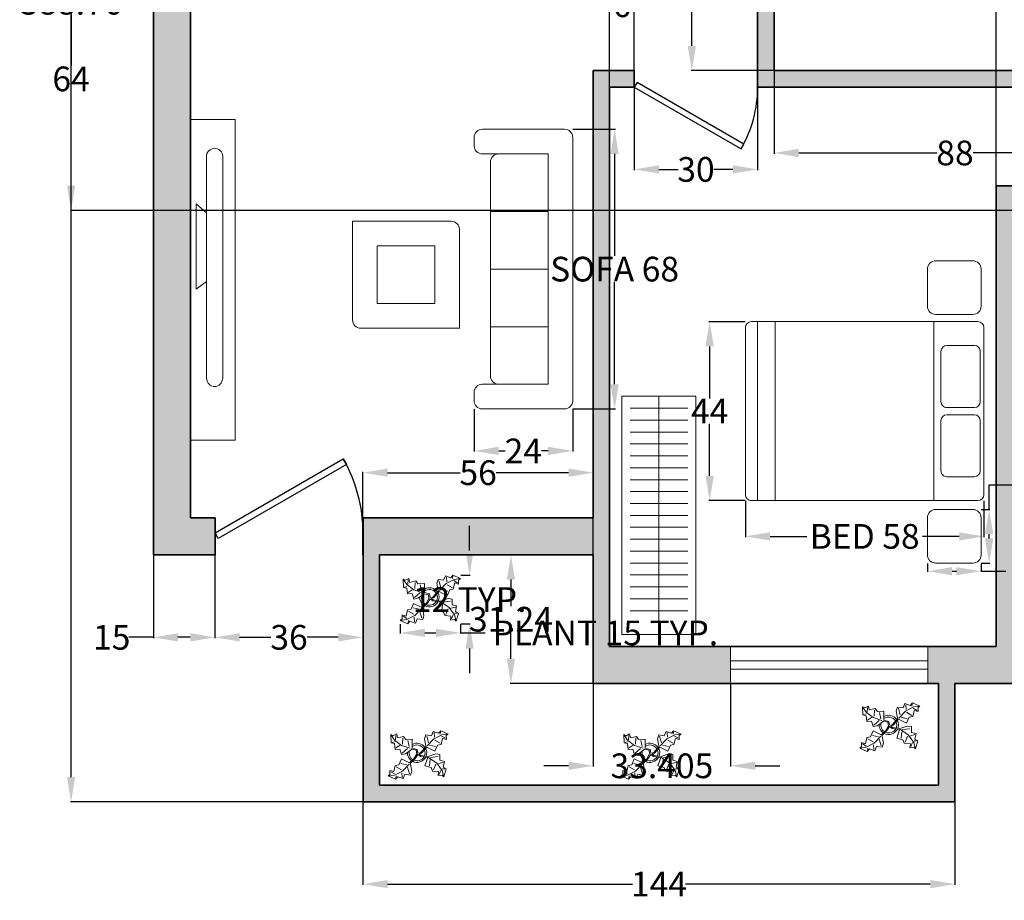
# Model space of a CAD drawing. Units: inches. Extents: x -26 to 363, y -399 to 37.
# Tile 1 of 4: x -7 to 232, y -399 to -185. Entities that reach past the tile are written whole.
import ezdxf

# ---------------------------------------------------------------- set-up
doc = ezdxf.new("R2010")
doc.units = ezdxf.units.IN
doc.header["$MEASUREMENT"] = 0
for name, color, linetype, lineweight in [('A-ANNO-DIMS', 2, 'Continuous', 18), ('A-DOOR', 3, 'Continuous', 25), ('A-EQPM', 9, 'Continuous', 18), ('A-FLOR-CASE', 8, 'Continuous', 18), ('A-FURN', 8, 'Continuous', 18), ('A-GLAZ', 4, 'Continuous', 18), ('A-WALL', 7, 'Continuous', 35), ('A-WALL-PATT', 251, 'Continuous', 13), ('L-PLNT', 94, 'Continuous', 13)]:
    doc.layers.add(name, color=color, linetype=linetype, lineweight=lineweight)
doc.styles.get("Standard").update_dxf_attribs({"font": 'arial.ttf'})
doc.dimstyles.get("Standard").update_dxf_attribs({"dimtxt": 6, "dimasz": 6, "dimexe": 0.18, "dimexo": 0.0625, "dimgap": 0.09, "dimtad": 0, "dimtih": 1, "dimtoh": 1, "dimdec": 0, "dimzin": 0, "dimdsep": 46, "dimlunit": 4, "dimtxsty": 'Standard', "dimcen": 0.09, "dimadec": 0, "dimazin": 0, "dimtfac": 1, "dimtdec": 0, "dimtofl": 0, "dimtmove": 0, "dimatfit": 3, "dimfxl": 1, "dimtolj": 1, "dimtzin": 0, "dimarcsym": 0})

# ---------------------------------------------------------------- blocks, each defined once
blk = doc.blocks.new('*U2')
for p, q in [((0, 0), (0, -6)), ((40, 0), (40, -6))]:
    blk.add_line(p, q)
blk.add_lwpolyline([(0, 0), (34.64, 20), (35.52, 18.48), (0.87, -1.52)], close=True)
blk.add_arc((0, 0), 40, 0, 30)
blk = doc.blocks.new('*U3')
for p, q in [((0, 0), (0, 6)), ((40, 0), (40, 6))]:
    blk.add_line(p, q)
blk.add_lwpolyline([(0, 0), (34.64, -20), (35.52, -18.48), (0.87, 1.52)], close=True)
blk.add_arc((0, 0), 40, 330, 0)
blk = doc.blocks.new('Bed - Queen')
for p, q in [((2, 0), (57.99999, 0)), ((0, -78.00003), (0, -2)), ((7.99999, -12.4), (7.99999, -3.2)), ((9.99999, -1.2), (26.79998, -1.2)), ((28.79998, -3.2), (28.79998, -12.4)), ((31.19999, -12.4), (31.19999, -3.2)), ((33.19999, -1.2), (49.99999, -1.2)), ((51.99999, -3.2), (51.99999, -12.4)), ((59.99999, -2), (59.99999, -78.00003)), ((9.99999, -14.4), (26.79998, -14.4)), ((33.19999, -14.4), (49.99999, -14.4)), ((59.99999, -16.8), (0, -16.8)), ((59.99999, -70.00003), (0, -70.00003)), ((59.99999, -76.00003), (0, -76.00003)), ((57.99999, -80.00003), (2, -80.00003))]:
    blk.add_line(p, q)
for centre, start, end in [((2, -2), 90, 180), ((57.99999, -2), 0, 90), ((9.99999, -3.2), 90, 180), ((26.79998, -3.2), 0, 90), ((33.19999, -3.2), 90, 180), ((49.99999, -3.2), 0, 90), ((9.99999, -12.4), 180, 270), ((26.79998, -12.4), 270, 0), ((33.19999, -12.4), 180, 270), ((49.99999, -12.4), 270, 0), ((2, -78.00003), 180, 270), ((57.99999, -78.00003), 270, 0)]:
    blk.add_arc(centre, 2, start, end)
blk = doc.blocks.new('SOFA')
for p, q in [((-21.98, 0), (-2, 0)), ((-23.96, -4.02), (-23.98, -2.02)), ((0, -2), (0, -62)), ((-6, -6), (-21.96, -6)), ((-6, -62), (-6, -6)), ((-22, -62), (-6, -62)), ((0, -62), (0, -66)), ((-24, -66), (-24, -64)), ((-2, -68), (-22, -68))]:
    blk.add_line(p, q)
for points in [[(-6, -6), (-18, -6, 0.414214), (-20, -8), (-20, -20), (-6, -20)], [(-6, -48), (-20, -48), (-20, -60, 0.414214), (-18, -62), (-6, -62)]]:
    blk.add_lwpolyline(points, format="xyb", close=True)
for points in [[(-6, -20), (-20, -20), (-20, -34), (-6, -34)], [(-6, -34), (-20, -34), (-20, -48), (-6, -48)]]:
    blk.add_lwpolyline(points, close=True)
for centre, start, end in [((-21.98, -2), 90, 180.5593), ((-2, -2), 0, 90), ((-21.96, -4), 180.5593, 270), ((-22, -64), 90, 180), ((-22, -66), 180, 270), ((-2, -66), 270, 360)]:
    blk.add_arc(centre, 2, start, end)
blk = doc.blocks.new('Plant - Rubber or Philodendron')
for p, q in [((8.8871, 10.7908), (9.9809, 13.4933)), ((9.9809, 13.4933), (13.3837, 12.301)), ((10.5828, 12.6946), (10.8893, 9.7953)), ((13.3837, 12.301), (14.68, 13.9039)), ((14.5816, 13.2037), (14.3848, 11.8033)), ((14.68, 13.9039), (19.3848, 11.8146)), ((-16.2005, 11.4774), (-13.9899, 8.1064)), ((-16.2005, 11.4774), (-14.8639, 10.7964)), ((-16.0159, 6.3329), (-16.2005, 11.4774)), ((-14.0069, 5.8704), (-16.0159, 6.3329)), ((-15.3434, 6.5514), (-13.9984, 6.9884)), ((-14.8639, 10.7964), (-12.6195, 11.8975)), ((-13.9899, 8.1064), (-9.5434, 4.7185)), ((-13.3174, 8.325), (-13.0735, 11.0065)), ((-12.6195, 11.8975), (-12.1909, 9.4345)), ((-12.1909, 9.4345), (-8.3829, 10.3)), ((-8.8369, 9.409), (-9.0894, 5.6095)), ((-8.3829, 10.3), (-7.0549, 8.501)), ((-7.0549, 8.501), (-3.0284, 8.6941)), ((-4.8529, 4.012), (-5.7184, 7.82)), ((-3.0284, 8.6941), (-3.0709, 3.1041)), ((4.6914, 8.8812), (5.3859, 11.2828)), ((4.6914, 8.8812), (5.5014, 4.4831)), ((5.3859, 11.2828), (8.8871, 10.7908)), ((5.9878, 10.4842), (7.1971, 6.3869)), ((10.3916, 8.7942), (6.2847, 4.4028)), ((15.3859, 11.3055), (10.3916, 8.7942)), ((14.2977, 6.1031), (10.9934, 7.9956)), ((15.7909, 9.1065), (14.8995, 5.3044)), ((15.2875, 10.6053), (17.5907, 9.2105)), ((19.3848, 11.8146), (15.3859, 11.3055)), ((18.1925, 8.4119), (15.7909, 9.1065)), ((19.3848, 11.8146), (18.1868, 10.9119)), ((18.1868, 10.9119), (18.1925, 8.4119)), ((-13.5868, 2.2894), (-14.0069, 5.8704)), ((-10.6784, 2.491), (-13.5868, 2.2894)), ((-13.1329, 3.1804), (-10.6614, 4.727)), ((-9.5858, -0.8715), (-10.6784, 2.491)), ((-9.5434, 4.7185), (-4.1917, 2.9888)), ((-9.1318, 0.0195), (-5.9793, 2.9025)), ((-7.1228, -0.443), (-3.5248, 2.2131)), ((-3.5248, 2.2131), (-3.3011, 2.4355)), ((-3.3011, 2.4355), (-0.5306, 1.7947)), ((-3.0709, 3.1041), (0.0797, 2.3163)), ((-0.5306, 1.7947), (-0.2255, -0.5527)), ((-0.5306, 1.7947), (-0.5306, 1.7947)), ((0.0797, 2.3163), (0.4866, -0.031)), ((0.4866, -0.031), (2.1141, 0.2298)), ((2.1141, 0.2298), (5.4346, 3.9146)), ((6.1032, 3.6844), (2.8262, -0.031)), ((5.4346, 3.9146), (5.5014, 4.4831)), ((11.1089, 1.1958), (6.1032, 3.6844)), ((7.7005, 4.8881), (11.5025, 3.9967)), ((12.7005, 4.8994), (11.1089, 1.1958)), ((14.8995, 5.3044), (12.7005, 4.8994)), ((-11.3237, -7.2629), (-9.7321, -3.5593)), ((-9.7321, -3.5593), (-4.7264, -6.0479)), ((-7.1228, -0.443), (-9.5858, -0.8715)), ((-2.019, -3.6148), (-4.7264, -6.0479)), ((-4.0579, -6.2781), (-0.9375, -3.1608)), ((-2.019, -3.6148), (-0.2255, -0.5527)), ((-0.9375, -3.1608), (0.5883, -0.8135)), ((0.5883, -0.8135), (2.2447, -2.0916)), ((2.8262, -0.031), (1.3003, -0.5527)), ((1.3003, -0.5527), (2.4193, -1.4655)), ((2.2447, -2.0916), (6.7108, -2.6626)), ((2.4193, -1.4655), (6.895, -2.1175)), ((4.943, -7.9659), (6.7108, -2.6626)), ((11.6605, -0.5413), (6.895, -2.1175)), ((12.3677, -6.1981), (7.219, -2.6772)), ((8.125, -4.0768), (7.7715, -7.9659)), ((8.3544, -2.7453), (13.1973, -2.1704)), ((11.6605, -0.5413), (14.1354, -0.8948)), ((16.2567, -5.8446), (13.4283, -6.5517)), ((14.1354, -0.8948), (14.1354, -4.4304)), ((14.1354, -4.4304), (16.9638, -5.1375)), ((16.9638, -5.1375), (16.2567, -8.673)), ((-16.8157, -10.7754), (-14.4141, -11.4699)), ((-16.8101, -13.2754), (-16.8157, -10.7754)), ((-13.9107, -12.9688), (-16.2139, -11.574)), ((-14.4141, -11.4699), (-13.5228, -7.6679)), ((-14.0091, -13.669), (-9.0148, -11.1577)), ((-13.5228, -7.6679), (-11.3237, -7.2629)), ((-12.921, -8.4665), (-9.6166, -10.359)), ((-6.3237, -7.2516), (-10.1257, -6.3602)), ((-9.206, -15.0581), (-9.5126, -12.1588)), ((-9.0148, -11.1577), (-4.9047, -6.8122)), ((-4.611, -12.8477), (-5.8203, -8.7504)), ((-4.1246, -6.8466), (-4.0579, -6.2781)), ((-3.3146, -11.2447), (-4.1246, -6.8466)), ((-3.3146, -11.2447), (-4.0092, -13.6463)), ((8.8321, -9.0266), (4.943, -7.9659)), ((9.5392, -11.1479), (8.8321, -9.0266)), ((13.4283, -11.5015), (9.5392, -11.1479)), ((10.2463, -10.4408), (11.6605, -6.9053)), ((15.5496, -10.7943), (12.3677, -6.1981)), ((13.0748, -13.9763), (13.4283, -11.5015)), ((14.8425, -10.7943), (13.7819, -13.2692)), ((16.6103, -14.6834), (15.5496, -10.7943)), ((17.3174, -9.7337), (15.9032, -9.7337)), ((16.2567, -8.673), (18.0245, -9.7337)), ((18.0245, -9.7337), (16.6103, -14.6834)), ((-18.008, -14.1781), (-16.8101, -13.2754)), ((-18.008, -14.1781), (-14.0091, -13.669)), ((-13.3032, -16.2674), (-18.008, -14.1781)), ((-12.0069, -14.6645), (-13.3032, -16.2674)), ((-13.2048, -15.5672), (-13.008, -14.1668)), ((-8.6042, -15.8568), (-12.0069, -14.6645)), ((-7.5103, -13.1543), (-8.6042, -15.8568)), ((-4.0092, -13.6463), (-7.5103, -13.1543)), ((15.5496, -13.6228), (13.0748, -13.9763)), ((16.6103, -14.6834), (15.5496, -13.6228))]:
    blk.add_line(p, q)
for centre, radius, start, end in [((0, 0), 6.1275, 34.37569, 120.1028), ((0.0308, 0.1664), 6, 178.6147, 235.1169), ((0.0308, 0.1664), 5, 168.1647, 238.6725), ((-0.0601, -0.2075), 5.2461, 33.82192, 124.9414), ((-0.2664, 0.1682), 5.2775, 338.4094, 20.03007), ((-0.098, 0.1364), 6.1288, 341.2017, 26.09184), ((-0.0234, 0.3825), 6.1492, 242.5812, 331.2714), ((-0.1102, 0.4886), 5.2883, 247.3711, 327.472)]:
    blk.add_arc(centre, radius, start, end)
blk = doc.blocks.new('WIN-48IN')
for p, q in [((0, 0), (0, 9)), ((48, 9), (48, 0)), ((48, 5.5), (0, 5.5)), ((48, 3.5), (0, 3.5))]:
    blk.add_line(p, q)
blk = doc.blocks.new('NIGHTSTAND-13IN')
blk.add_lwpolyline([(11.05, 0), (2, 0, -0.414214), (0, 2), (0, 11.05, -0.414214), (2, 13.05), (11.05, 13.05, -0.414214), (13.05, 11.05), (13.05, 2, -0.414214)], format="xyb", close=True)
blk = doc.blocks.new('*D15')
at = {"layer": 'A-ANNO-DIMS', "color": 0, "lineweight": -2, "transparency": 16777216}
for p, q in [((85.4, -332.11), (85.4, -334.43)), ((100.05, -332.11), (100.05, -334.43)), ((91.4, -334.25), (94.05, -334.25)), ((100.05, -334.25), (106.05, -334.25))]:
    blk.add_line(p, q, dxfattribs=at)
at = {"layer": 'A-ANNO-DIMS', "color": 0, "transparency": 16777216}
for points in [[(91.4, -333.25), (91.4, -335.25), (85.4, -334.25)], [(94.05, -333.25), (94.05, -335.25), (100.05, -334.25)]]:
    blk.add_solid(points, dxfattribs=at)
at = {"layer": 'Defpoints', "color": 0, "transparency": 16777216}
for p in [(85.4, -332.05), (100.05, -332.05), (100.05, -334.25)]:
    blk.add_point(p, dxfattribs=at)
at = {"layer": 'A-ANNO-DIMS', "color": 0, "transparency": 16777216, "insert": (135.27, -334.25), "char_height": 6, "attachment_point": 5}
blk.add_mtext('\\A1;PLANT 15 TYP.', dxfattribs=at)
blk = doc.blocks.new('*D16')
at = {"layer": 'A-ANNO-DIMS', "color": 0, "lineweight": -2, "transparency": 16777216}
for p, q in [((102.25, -314.22), (102.25, -308.22)), ((100.11, -320.22), (102.43, -320.22)), ((100.11, -332.05), (102.43, -332.05)), ((102.25, -338.05), (102.25, -344.05))]:
    blk.add_line(p, q, dxfattribs=at)
at = {"layer": 'A-ANNO-DIMS', "color": 0, "transparency": 16777216}
for points in [[(101.25, -314.22), (103.25, -314.22), (102.25, -320.22)], [(101.25, -338.05), (103.25, -338.05), (102.25, -332.05)]]:
    blk.add_solid(points, dxfattribs=at)
at = {"layer": 'Defpoints', "color": 0, "transparency": 16777216}
for p in [(100.05, -320.22), (102.25, -320.22), (100.05, -332.05)]:
    blk.add_point(p, dxfattribs=at)
at = {"layer": 'A-ANNO-DIMS', "color": 0, "transparency": 16777216, "insert": (102.25, -326.14), "char_height": 6, "attachment_point": 5}
blk.add_mtext('\\A1;12 TYP.', dxfattribs=at)
blk = doc.blocks.new('*D19')
at = {"layer": 'A-ANNO-DIMS', "color": 0, "lineweight": -2, "transparency": 16777216}
for p, q in [((169.35, -302.15), (169.35, -310.97)), ((227.36, -302.15), (227.36, -310.97)), ((175.35, -310.79), (184.31, -310.79)), ((221.36, -310.79), (212.4, -310.79))]:
    blk.add_line(p, q, dxfattribs=at)
at = {"layer": 'A-ANNO-DIMS', "color": 0, "transparency": 16777216}
for points in [[(175.35, -309.79), (175.35, -311.79), (169.35, -310.79)], [(221.36, -309.79), (221.36, -311.79), (227.36, -310.79)]]:
    blk.add_solid(points, dxfattribs=at)
at = {"layer": 'Defpoints', "color": 0, "transparency": 16777216}
for p in [(169.35, -302.09), (227.36, -302.09), (227.36, -310.79)]:
    blk.add_point(p, dxfattribs=at)
at = {"layer": 'A-ANNO-DIMS', "color": 0, "transparency": 16777216, "insert": (198.36, -310.79), "char_height": 6, "attachment_point": 5}
blk.add_mtext('\\A1;BED 58', dxfattribs=at)
blk = doc.blocks.new('*D20')
at = {"layer": 'A-ANNO-DIMS', "color": 0, "lineweight": -2, "transparency": 16777216}
for p, q in [((169.29, -258.59), (160.47, -258.59)), ((160.65, -264.59), (160.65, -277.25)), ((160.65, -296.09), (160.65, -283.43)), ((169.29, -302.09), (160.47, -302.09))]:
    blk.add_line(p, q, dxfattribs=at)
at = {"layer": 'A-ANNO-DIMS', "color": 0, "transparency": 16777216}
for points in [[(159.65, -264.59), (161.65, -264.59), (160.65, -258.59)], [(159.65, -296.09), (161.65, -296.09), (160.65, -302.09)]]:
    blk.add_solid(points, dxfattribs=at)
at = {"layer": 'Defpoints', "color": 0, "transparency": 16777216}
for p in [(169.35, -258.59), (160.65, -302.09), (169.35, -302.09)]:
    blk.add_point(p, dxfattribs=at)
at = {"layer": 'A-ANNO-DIMS', "color": 0, "transparency": 16777216, "insert": (160.65, -280.34), "char_height": 6, "attachment_point": 5}
blk.add_mtext('\\A1;44', dxfattribs=at)
blk = doc.blocks.new('*D31')
at = {"layer": 'A-ANNO-DIMS', "color": 0, "lineweight": -2, "transparency": 16777216}
for p, q in [((213.62, -317.36), (213.62, -319.44)), ((226.67, -317.36), (226.67, -319.44)), ((219.62, -319.26), (220.67, -319.26)), ((226.67, -319.26), (232.67, -319.26))]:
    blk.add_line(p, q, dxfattribs=at)
at = {"layer": 'A-ANNO-DIMS', "color": 0, "transparency": 16777216}
for points in [[(219.62, -318.26), (219.62, -320.26), (213.62, -319.26)], [(220.67, -318.26), (220.67, -320.26), (226.67, -319.26)]]:
    blk.add_solid(points, dxfattribs=at)
at = {"layer": 'Defpoints', "color": 0, "transparency": 16777216}
for p in [(213.62, -317.3), (226.67, -317.3), (226.67, -319.26)]:
    blk.add_point(p, dxfattribs=at)
at = {"layer": 'A-ANNO-DIMS', "color": 0, "transparency": 16777216, "insert": (275.62, -319.26), "char_height": 6, "attachment_point": 5}
blk.add_mtext('\\A1;NIGHTSTAND 13 TYP.', dxfattribs=at)
blk = doc.blocks.new('*D32')
at = {"layer": 'A-ANNO-DIMS', "color": 0, "lineweight": -2, "transparency": 16777216}
for p, q in [((228.63, -304.25), (228.63, -298.25)), ((228.63, -298.25), (234.63, -298.25)), ((226.73, -304.25), (228.81, -304.25)), ((228.63, -311.3), (228.63, -310.25)), ((226.73, -317.3), (228.81, -317.3))]:
    blk.add_line(p, q, dxfattribs=at)
at = {"layer": 'A-ANNO-DIMS', "color": 0, "transparency": 16777216}
for points in [[(227.63, -310.25), (229.63, -310.25), (228.63, -304.25)], [(227.63, -311.3), (229.63, -311.3), (228.63, -317.3)]]:
    blk.add_solid(points, dxfattribs=at)
at = {"layer": 'Defpoints', "color": 0, "transparency": 16777216}
for p in [(226.67, -304.25), (228.63, -304.25), (226.67, -317.3)]:
    blk.add_point(p, dxfattribs=at)
at = {"layer": 'A-ANNO-DIMS', "color": 0, "transparency": 16777216, "insert": (249.04, -298.25), "char_height": 6, "attachment_point": 5}
blk.add_mtext('\\A1;13 TYP.', dxfattribs=at)
blk = doc.blocks.new('*D37')
at = {"layer": 'A-ANNO-DIMS', "color": 0, "lineweight": -2, "transparency": 16777216}
for p, q in [((127.39, -211.81), (137.71, -211.81)), ((137.53, -217.81), (137.53, -242.61)), ((137.53, -273.81), (137.53, -249)), ((127.39, -279.81), (137.71, -279.81))]:
    blk.add_line(p, q, dxfattribs=at)
at = {"layer": 'A-ANNO-DIMS', "color": 0, "transparency": 16777216}
for points in [[(136.53, -217.81), (138.53, -217.81), (137.53, -211.81)], [(136.53, -273.81), (138.53, -273.81), (137.53, -279.81)]]:
    blk.add_solid(points, dxfattribs=at)
at = {"layer": 'Defpoints', "color": 0, "transparency": 16777216}
for p in [(127.33, -211.81), (137.53, -211.81), (127.33, -279.81)]:
    blk.add_point(p, dxfattribs=at)
at = {"layer": 'A-ANNO-DIMS', "color": 0, "transparency": 16777216, "insert": (137.53, -245.81), "char_height": 6, "attachment_point": 5}
blk.add_mtext('\\A1;SOFA 68', dxfattribs=at)
blk = doc.blocks.new('*D38')
at = {"layer": 'A-ANNO-DIMS', "color": 0, "lineweight": -2, "transparency": 16777216}
for p, q in [((103.33, -279.87), (103.33, -290.19)), ((127.33, -279.87), (127.33, -290.19)), ((109.33, -290.01), (110.9, -290.01)), ((121.33, -290.01), (119.76, -290.01))]:
    blk.add_line(p, q, dxfattribs=at)
at = {"layer": 'A-ANNO-DIMS', "color": 0, "transparency": 16777216}
for points in [[(109.33, -289.01), (109.33, -291.01), (103.33, -290.01)], [(121.33, -289.01), (121.33, -291.01), (127.33, -290.01)]]:
    blk.add_solid(points, dxfattribs=at)
at = {"layer": 'Defpoints', "color": 0, "transparency": 16777216}
for p in [(103.33, -279.81), (127.33, -279.81), (127.33, -290.01)]:
    blk.add_point(p, dxfattribs=at)
at = {"layer": 'A-ANNO-DIMS', "color": 0, "transparency": 16777216, "insert": (115.33, -290.01), "char_height": 6, "attachment_point": 5}
blk.add_mtext('\\A1;24', dxfattribs=at)
blk = doc.blocks.new('*D40')
at = {"layer": 'A-ANNO-DIMS', "color": 0, "lineweight": -2, "transparency": 16777216}
for p, q in [((25.26, 13.44), (5.13, 13.44)), ((5.31, 7.44), (5.31, -177.78)), ((5.31, -369.31), (5.31, -184.09)), ((76.26, -375.31), (5.13, -375.31))]:
    blk.add_line(p, q, dxfattribs=at)
at = {"layer": 'A-ANNO-DIMS', "color": 0, "transparency": 16777216}
for points in [[(4.31, 7.44), (6.31, 7.44), (5.31, 13.44)], [(4.31, -369.31), (6.31, -369.31), (5.31, -375.31)]]:
    blk.add_solid(points, dxfattribs=at)
at = {"layer": 'Defpoints', "color": 0, "transparency": 16777216}
for p in [(25.32, 13.44), (5.31, -375.31), (76.32, -375.31)]:
    blk.add_point(p, dxfattribs=at)
at = {"layer": 'A-ANNO-DIMS', "color": 0, "transparency": 16777216, "insert": (5.31, -180.93), "char_height": 6, "attachment_point": 5}
blk.add_mtext('\\A1;388.76', dxfattribs=at)
blk = doc.blocks.new('*D42')
at = {"layer": 'A-ANNO-DIMS', "color": 0, "lineweight": -2, "transparency": 16777216}
for p, q in [((25.32, -315.38), (25.32, -335.51)), ((40.32, -315.38), (40.32, -335.51)), ((25.32, -335.33), (19.32, -335.33)), ((34.32, -335.33), (31.32, -335.33))]:
    blk.add_line(p, q, dxfattribs=at)
at = {"layer": 'A-ANNO-DIMS', "color": 0, "transparency": 16777216}
for points in [[(31.32, -334.33), (31.32, -336.33), (25.32, -335.33)], [(34.32, -334.33), (34.32, -336.33), (40.32, -335.33)]]:
    blk.add_solid(points, dxfattribs=at)
at = {"layer": 'Defpoints', "color": 0, "transparency": 16777216}
for p in [(25.32, -315.31), (40.32, -315.31), (25.32, -335.33)]:
    blk.add_point(p, dxfattribs=at)
at = {"layer": 'A-ANNO-DIMS', "color": 0, "transparency": 16777216, "insert": (15.2, -335.33), "char_height": 6, "attachment_point": 5}
blk.add_mtext('\\A1;15', dxfattribs=at)
blk = doc.blocks.new('*D43')
at = {"layer": 'A-ANNO-DIMS', "color": 0, "lineweight": -2, "transparency": 16777216}
for p, q in [((76.32, -375.38), (76.32, -395.51)), ((220.32, -375.38), (220.32, -395.51)), ((82.32, -395.33), (141.9, -395.33)), ((214.32, -395.33), (154.75, -395.33))]:
    blk.add_line(p, q, dxfattribs=at)
at = {"layer": 'A-ANNO-DIMS', "color": 0, "transparency": 16777216}
for points in [[(82.32, -394.33), (82.32, -396.33), (76.32, -395.33)], [(214.32, -394.33), (214.32, -396.33), (220.32, -395.33)]]:
    blk.add_solid(points, dxfattribs=at)
at = {"layer": 'Defpoints', "color": 0, "transparency": 16777216}
for p in [(76.32, -375.31), (220.32, -375.31), (220.32, -395.33)]:
    blk.add_point(p, dxfattribs=at)
at = {"layer": 'A-ANNO-DIMS', "color": 0, "transparency": 16777216, "insert": (148.32, -395.33), "char_height": 6, "attachment_point": 5}
blk.add_mtext('\\A1;144', dxfattribs=at)
blk = doc.blocks.new('*D44')
at = {"layer": 'A-ANNO-DIMS', "color": 0, "lineweight": -2, "transparency": 16777216}
for p, q in [((132.26, -315.31), (112.13, -315.31)), ((112.31, -321.31), (112.31, -327.78)), ((112.31, -340.56), (112.31, -334.09)), ((132.26, -346.56), (112.13, -346.56))]:
    blk.add_line(p, q, dxfattribs=at)
at = {"layer": 'A-ANNO-DIMS', "color": 0, "transparency": 16777216}
for points in [[(111.31, -321.31), (113.31, -321.31), (112.31, -315.31)], [(111.31, -340.56), (113.31, -340.56), (112.31, -346.56)]]:
    blk.add_solid(points, dxfattribs=at)
at = {"layer": 'Defpoints', "color": 0, "transparency": 16777216}
for p in [(112.31, -315.31), (132.32, -315.31), (132.32, -346.56)]:
    blk.add_point(p, dxfattribs=at)
at = {"layer": 'A-ANNO-DIMS', "color": 0, "transparency": 16777216, "insert": (112.31, -330.93), "char_height": 6, "attachment_point": 5}
blk.add_mtext('\\A1;31.24', dxfattribs=at)
blk = doc.blocks.new('*D47')
at = {"layer": 'A-ANNO-DIMS', "color": 0, "lineweight": -2, "transparency": 16777216}
for p, q in [((176.32, -197.62), (176.32, -217.75)), ((264.32, -197.62), (264.32, -217.75)), ((182.32, -217.57), (215.93, -217.57)), ((258.32, -217.57), (224.72, -217.57))]:
    blk.add_line(p, q, dxfattribs=at)
at = {"layer": 'A-ANNO-DIMS', "color": 0, "transparency": 16777216}
for points in [[(182.32, -216.57), (182.32, -218.57), (176.32, -217.57)], [(258.32, -216.57), (258.32, -218.57), (264.32, -217.57)]]:
    blk.add_solid(points, dxfattribs=at)
at = {"layer": 'Defpoints', "color": 0, "transparency": 16777216}
for p in [(176.32, -197.56), (264.32, -197.56), (176.32, -217.57)]:
    blk.add_point(p, dxfattribs=at)
at = {"layer": 'A-ANNO-DIMS', "color": 0, "transparency": 16777216, "insert": (220.32, -217.57), "char_height": 6, "attachment_point": 5}
blk.add_mtext('\\A1;88', dxfattribs=at)
blk = doc.blocks.new('*D48')
at = {"layer": 'A-ANNO-DIMS', "color": 0, "lineweight": -2, "transparency": 16777216}
for p, q in [((176.26, -91.56), (156.13, -91.56)), ((156.31, -97.56), (156.31, -141.4)), ((156.31, -191.56), (156.31, -147.71)), ((176.26, -197.56), (156.13, -197.56))]:
    blk.add_line(p, q, dxfattribs=at)
at = {"layer": 'A-ANNO-DIMS', "color": 0, "transparency": 16777216}
for points in [[(155.31, -97.56), (157.31, -97.56), (156.31, -91.56)], [(155.31, -191.56), (157.31, -191.56), (156.31, -197.56)]]:
    blk.add_solid(points, dxfattribs=at)
at = {"layer": 'Defpoints', "color": 0, "transparency": 16777216}
for p in [(156.31, -91.56), (176.32, -91.56), (176.32, -197.56)]:
    blk.add_point(p, dxfattribs=at)
at = {"layer": 'A-ANNO-DIMS', "color": 0, "transparency": 16777216, "insert": (156.31, -144.56), "char_height": 6, "attachment_point": 5}
blk.add_mtext('\\A1;106', dxfattribs=at)
blk = doc.blocks.new('*D51')
at = {"layer": 'A-ANNO-DIMS', "color": 0, "lineweight": -2, "transparency": 16777216}
for p, q in [((268.26, -167.56), (5.13, -167.56)), ((5.31, -173.56), (5.31, -196.4)), ((5.31, -225.56), (5.31, -202.71)), ((268.26, -231.56), (5.13, -231.56))]:
    blk.add_line(p, q, dxfattribs=at)
at = {"layer": 'A-ANNO-DIMS', "color": 0, "transparency": 16777216}
for points in [[(4.31, -173.56), (6.31, -173.56), (5.31, -167.56)], [(4.31, -225.56), (6.31, -225.56), (5.31, -231.56)]]:
    blk.add_solid(points, dxfattribs=at)
at = {"layer": 'Defpoints', "color": 0, "transparency": 16777216}
for p in [(268.32, -167.56), (5.31, -231.56), (268.32, -231.56)]:
    blk.add_point(p, dxfattribs=at)
at = {"layer": 'A-ANNO-DIMS', "color": 0, "transparency": 16777216, "insert": (5.31, -199.56), "char_height": 6, "attachment_point": 5}
blk.add_mtext('\\A1;64', dxfattribs=at)
blk = doc.blocks.new('*D55')
at = {"layer": 'A-ANNO-DIMS', "color": 0, "lineweight": -2, "transparency": 16777216}
for p, q in [((132.32, -346.62), (132.32, -366.75)), ((165.73, -346.62), (165.73, -366.75)), ((126.32, -366.57), (120.32, -366.57)), ((171.73, -366.57), (177.73, -366.57))]:
    blk.add_line(p, q, dxfattribs=at)
at = {"layer": 'A-ANNO-DIMS', "color": 0, "transparency": 16777216}
for points in [[(126.32, -365.57), (126.32, -367.57), (132.32, -366.57)], [(171.73, -365.57), (171.73, -367.57), (165.73, -366.57)]]:
    blk.add_solid(points, dxfattribs=at)
at = {"layer": 'Defpoints', "color": 0, "transparency": 16777216}
for p in [(132.32, -346.56), (165.73, -346.56), (132.32, -366.57)]:
    blk.add_point(p, dxfattribs=at)
at = {"layer": 'A-ANNO-DIMS', "color": 0, "transparency": 16777216, "insert": (149.03, -366.57), "char_height": 6, "attachment_point": 5}
blk.add_mtext('\\A1;33.405', dxfattribs=at)
blk = doc.blocks.new('*D59')
at = {"layer": 'A-ANNO-DIMS', "color": 0, "lineweight": -2, "transparency": 16777216}
for p, q in [((40.32, -315.38), (40.32, -335.51)), ((76.32, -315.38), (76.32, -335.51)), ((46.32, -335.33), (53.94, -335.33)), ((70.32, -335.33), (62.71, -335.33))]:
    blk.add_line(p, q, dxfattribs=at)
at = {"layer": 'A-ANNO-DIMS', "color": 0, "transparency": 16777216}
for points in [[(46.32, -334.33), (46.32, -336.33), (40.32, -335.33)], [(70.32, -334.33), (70.32, -336.33), (76.32, -335.33)]]:
    blk.add_solid(points, dxfattribs=at)
at = {"layer": 'Defpoints', "color": 0, "transparency": 16777216}
for p in [(40.32, -315.31), (76.32, -315.31), (40.32, -335.33)]:
    blk.add_point(p, dxfattribs=at)
at = {"layer": 'A-ANNO-DIMS', "color": 0, "transparency": 16777216, "insert": (58.32, -335.33), "char_height": 6, "attachment_point": 5}
blk.add_mtext('\\A1;36', dxfattribs=at)
blk = doc.blocks.new('*D70')
at = {"layer": 'A-ANNO-DIMS', "color": 0, "lineweight": -2, "transparency": 16777216}
for p, q in [((142.32, -201.62), (142.32, -221.75)), ((172.32, -201.62), (172.32, -221.75)), ((148.32, -221.57), (152.95, -221.57)), ((166.32, -221.57), (161.7, -221.57))]:
    blk.add_line(p, q, dxfattribs=at)
at = {"layer": 'A-ANNO-DIMS', "color": 0, "transparency": 16777216}
for points in [[(148.32, -220.57), (148.32, -222.57), (142.32, -221.57)], [(166.32, -220.57), (166.32, -222.57), (172.32, -221.57)]]:
    blk.add_solid(points, dxfattribs=at)
at = {"layer": 'Defpoints', "color": 0, "transparency": 16777216}
for p in [(142.32, -201.56), (172.32, -201.56), (142.32, -221.57)]:
    blk.add_point(p, dxfattribs=at)
at = {"layer": 'A-ANNO-DIMS', "color": 0, "transparency": 16777216, "insert": (157.32, -221.57), "char_height": 6, "attachment_point": 5}
blk.add_mtext('\\A1;30', dxfattribs=at)
blk = doc.blocks.new('*D71')
at = {"layer": 'A-ANNO-DIMS', "color": 0, "lineweight": -2, "transparency": 16777216}
for p, q in [((130.322775, -181.538613), (124.322775, -181.538613)), ((136.322775, -201.492613), (136.322775, -181.358613)), ((142.322775, -201.492613), (142.322775, -181.358613)), ((148.322775, -181.538613), (154.322775, -181.538613))]:
    blk.add_line(p, q, dxfattribs=at)
at = {"layer": 'A-ANNO-DIMS', "color": 0, "transparency": 16777216}
for points in [[(130.322775, -180.538613), (130.322775, -182.538613), (136.322775, -181.538613)], [(148.322775, -180.538613), (148.322775, -182.538613), (142.322775, -181.538613)]]:
    blk.add_solid(points, dxfattribs=at)
at = {"layer": 'Defpoints', "color": 0, "transparency": 16777216}
for p in [(142.322775, -181.538613), (136.322775, -201.555113), (142.322775, -201.555113)]:
    blk.add_point(p, dxfattribs=at)
at = {"layer": 'A-ANNO-DIMS', "color": 0, "transparency": 16777216, "insert": (139.322775, -181.538613), "char_height": 6, "attachment_point": 5}
blk.add_mtext('\\A1;6', dxfattribs=at)
blk = doc.blocks.new('*D75')
at = {"layer": 'A-ANNO-DIMS', "color": 0, "lineweight": -2, "transparency": 16777216}
for p, q in [((76.32, -315.25), (76.32, -295.12)), ((82.32, -295.3), (99.94, -295.3)), ((126.32, -295.3), (108.71, -295.3)), ((132.32, -315.25), (132.32, -295.12))]:
    blk.add_line(p, q, dxfattribs=at)
at = {"layer": 'A-ANNO-DIMS', "color": 0, "transparency": 16777216}
for points in [[(82.32, -294.3), (82.32, -296.3), (76.32, -295.3)], [(126.32, -294.3), (126.32, -296.3), (132.32, -295.3)]]:
    blk.add_solid(points, dxfattribs=at)
at = {"layer": 'Defpoints', "color": 0, "transparency": 16777216}
for p in [(132.32, -295.3), (76.32, -315.31), (132.32, -315.31)]:
    blk.add_point(p, dxfattribs=at)
at = {"layer": 'A-ANNO-DIMS', "color": 0, "transparency": 16777216, "insert": (104.32, -295.3), "char_height": 6, "attachment_point": 5}
blk.add_mtext('\\A1;56', dxfattribs=at)
blk = doc.blocks.new('*D76')
at = {"layer": 'A-ANNO-DIMS', "color": 0, "lineweight": -2, "transparency": 16777216}
for p, q in [((136.32, -337.49), (136.32, 33.64)), ((230.32, -337.49), (230.32, 33.64)), ((142.32, 33.46), (178.95, 33.46)), ((224.32, 33.46), (187.7, 33.46))]:
    blk.add_line(p, q, dxfattribs=at)
at = {"layer": 'A-ANNO-DIMS', "color": 0, "transparency": 16777216}
for points in [[(142.32, 34.46), (142.32, 32.46), (136.32, 33.46)], [(224.32, 34.46), (224.32, 32.46), (230.32, 33.46)]]:
    blk.add_solid(points, dxfattribs=at)
at = {"layer": 'Defpoints', "color": 0, "transparency": 16777216}
for p in [(230.32, 33.46), (136.32, -337.56), (230.32, -337.56)]:
    blk.add_point(p, dxfattribs=at)
at = {"layer": 'A-ANNO-DIMS', "color": 0, "transparency": 16777216, "insert": (183.32, 33.46), "char_height": 6, "attachment_point": 5}
blk.add_mtext('\\A1;94', dxfattribs=at)

msp = doc.modelspace()

# ---------------------------------------------------------------- hatches: boundary and pattern name
at = {"layer": 'A-WALL-PATT'}
h = msp.add_hatch(color=256, dxfattribs=at)
h.dxf.hatch_style = 1
h.paths.add_polyline_path([(34.3228, -91.5551), (90.3228, -91.5551), (90.3228, -87.5551), (34.3228, -87.5551), (34.3228, 4.4449), (67.429, 4.4449), (67.429, 13.4449), (25.3228, 13.4449), (25.3228, -315.3126), (34.3228, -315.3126), (40.3228, -315.3126), (40.3228, -306.3126), (34.3228, -306.3126)])
h = msp.add_hatch(color=256, dxfattribs=at)
h.dxf.hatch_style = 1
h.paths.add_polyline_path([(325.3228, -139.9712), (316.3228, -139.9712), (316.3228, -163.5551), (292.3228, -163.5551), (268.3228, -163.5551), (268.3228, -91.5551), (274.3228, -91.5551), (274.3228, -87.5551), (172.3228, -87.5551), (172.3228, -91.5551), (172.3228, -97.5551), (176.3228, -97.5551), (176.3228, -91.5551), (264.3228, -91.5551), (264.3228, -197.5551), (258.3228, -197.5551), (176.3228, -197.5551), (176.3228, -127.5551), (172.3228, -127.5551), (172.3228, -197.5551), (172.3228, -201.5551), (258.3228, -201.5551), (264.3228, -201.5551), (268.3228, -201.5551), (268.3228, -167.5551), (316.3228, -167.5551), (316.3228, -187.2842), (325.3228, -187.2842)])
h = msp.add_hatch(color=256, dxfattribs=at)
h.dxf.hatch_style = 1
h.paths.add_polyline_path([(255.0334, -337.5551), (234.3228, -337.5551), (234.3228, -225.5551), (230.3228, -225.5551), (230.3228, -337.5551), (213.7273, -337.5551), (213.7273, -346.5551), (216.3228, -346.5551), (216.3228, -371.3126), (80.3228, -371.3126), (80.3228, -315.3126), (132.3228, -315.3126), (132.3228, -337.5551), (132.3228, -346.5551), (165.7273, -346.5551), (165.7273, -337.5551), (136.3228, -337.5551), (136.3228, -201.5551), (142.3228, -201.5551), (142.3228, -197.5551), (132.3228, -197.5551), (132.3228, -306.3126), (76.3228, -306.3126), (76.3228, -315.3126), (76.3228, -375.3126), (220.3228, -375.3126), (220.3228, -346.5551), (255.0334, -346.5551)])

# ---------------------------------------------------------------- linework, layer by layer
at = {"layer": 'A-EQPM'}
msp.add_line((35.7382, -250.7062), (38.2543, -248.7962), dxfattribs=at)
for points in [[(38.327, -272.4497), (38.2543, -272.4497), (38.2543, -218.4597)], [(42.2092, -218.4597), (42.2092, -272.4497), (42.1366, -272.4497)], [(35.7382, -250.7062), (35.7382, -229.9456), (38.2543, -232.1185)], [(38.2543, -229.9456), (38.2543, -250.7062)]]:
    msp.add_lwpolyline(points, dxfattribs=at)
for centre, radius, start, end in [((40.2318, -218.4597), 2.0188, 348.379925, 191.620075), ((40.2318, -272.4497), 1.9048, 180, 0)]:
    msp.add_arc(centre, radius, start, end, dxfattribs=at)
at = {"layer": 'A-FLOR-CASE'}
for p, q in [((141.3088, -276.7275), (155.3088, -276.7275)), ((148.3088, -276.7275), (148.3088, -331.762)), ((141.3088, -279.6241), (155.3088, -279.6241)), ((141.3088, -282.5206), (155.3088, -282.5206)), ((141.3088, -285.4172), (155.3088, -285.4172)), ((141.3088, -288.3137), (155.3088, -288.3137)), ((141.3088, -291.2103), (155.3088, -291.2103)), ((141.3088, -294.1068), (155.3088, -294.1068)), ((141.3088, -297.0034), (155.3088, -297.0034)), ((141.3088, -299.8999), (155.3088, -299.8999)), ((141.3088, -302.7965), (155.3088, -302.7965)), ((141.3088, -305.693), (155.3088, -305.693)), ((141.3088, -308.5896), (155.3088, -308.5896)), ((141.3088, -311.4861), (155.3088, -311.4861)), ((141.3088, -314.3827), (155.3088, -314.3827)), ((141.3088, -317.2793), (155.3088, -317.2793)), ((141.3088, -320.1758), (155.3088, -320.1758)), ((141.3088, -323.0724), (155.3088, -323.0724)), ((141.3088, -325.9689), (155.3088, -325.9689)), ((141.3088, -328.8655), (155.3088, -328.8655))]:
    msp.add_line(p, q, dxfattribs=at)
msp.add_lwpolyline([(157.3088, -334.6586), (157.3088, -276.7275), (139.3088, -276.7275), (139.3088, -334.6586), (157.3088, -334.6586), (139.3088, -334.6586)], dxfattribs=at)
at = {"layer": 'A-FURN'}
for points in [[(34.3228, -209.4703), (45.2602, -209.4703), (45.2602, -287.4025), (34.3228, -287.4025)], [(93.7863, -240.1794), (79.7863, -240.1794), (79.7863, -254.1794), (93.7863, -254.1794)]]:
    msp.add_lwpolyline(points, close=True, dxfattribs=at)
msp.add_lwpolyline([(97.7863, -234.1794), (73.7863, -234.1794), (73.7863, -258.1794, 0.41421356), (75.7863, -260.1794), (99.7863, -260.1794), (99.7863, -236.1794, 0.41421356)], format="xyb", close=True, dxfattribs=at)
at = {"layer": 'A-WALL'}
for p, q in [((34.3228, -306.3126), (34.3228, -91.5551)), ((172.3228, -197.5551), (172.3228, -127.5551)), ((176.3228, -197.5551), (176.3228, -127.5551)), ((132.3228, -197.5551), (132.3228, -306.3126)), ((142.3228, -197.5551), (132.3228, -197.5551)), ((142.3228, -201.5551), (142.3228, -197.5551)), ((172.3228, -201.5551), (172.3228, -197.5551)), ((258.3228, -197.5551), (176.3228, -197.5551)), ((136.3228, -201.5551), (136.3228, -337.5551)), ((142.3228, -201.5551), (136.3228, -201.5551)), ((258.3228, -201.5551), (172.3228, -201.5551)), ((230.3228, -225.5551), (230.3228, -337.5551)), ((234.3228, -225.5551), (230.3228, -225.5551)), ((40.3228, -306.3126), (34.3228, -306.3126)), ((40.3228, -306.3126), (40.3228, -315.3126)), ((76.3228, -306.3126), (76.3228, -315.3126)), ((132.3228, -306.3126), (76.3228, -306.3126)), ((34.3228, -315.3126), (25.3228, -315.3126)), ((40.3228, -315.3126), (34.3228, -315.3126)), ((76.3228, -315.3126), (76.3228, -375.3126)), ((132.3228, -315.3126), (80.3228, -315.3126)), ((80.3228, -315.3126), (80.3228, -371.3126)), ((132.3228, -315.3126), (132.3228, -337.5551)), ((132.3228, -337.5551), (132.3228, -346.5551)), ((230.3228, -337.5551), (136.3228, -337.5551)), ((216.3228, -371.3126), (216.3228, -346.5551)), ((220.3228, -375.3126), (220.3228, -346.5551)), ((80.3228, -371.3126), (216.3228, -371.3126)), ((76.3228, -375.3126), (220.3228, -375.3126))]:
    msp.add_line(p, q, dxfattribs=at)
for points in [[(25.3228, -315.3126), (25.3228, 13.4449), (325.3228, 13.4449), (325.3228, -346.5551), (220.3228, -346.5551)], [(216.3228, -346.5551), (132.3228, -346.5551)]]:
    msp.add_lwpolyline(points, dxfattribs=at)

# ---------------------------------------------------------------- block references
at = {"layer": 'A-DOOR'}
for name, p, xscale, yscale, zscale in [('*U3', (142.3228, -201.5551), 0.75, 0.75, 0.75), ('*U2', (40.3228, -309.9126), 0.9, 0.9, 0.9)]:
    msp.add_blockref(name, p, dxfattribs=dict(at, xscale=xscale, yscale=yscale, zscale=zscale))
at = {"layer": 'A-FURN'}
for name, p in [('SOFA', (127.3312, -211.805)), ('NIGHTSTAND-13IN', (213.62, -256.836)), ('NIGHTSTAND-13IN', (213.62, -317.2979))]:
    msp.add_blockref(name, p, dxfattribs=at)
at = {"layer": 'A-FURN', "xscale": 0.725065064120784, "yscale": 0.725065064120784, "zscale": 0.725065064120784, "rotation": 270}
msp.add_blockref('Bed - Queen', (227.3595, -258.5861), dxfattribs=at)
at = {"layer": 'A-GLAZ'}
msp.add_blockref('WIN-48IN', (165.7273, -346.555), dxfattribs=at)
at = {"layer": 'L-PLNT', "xscale": 0.3918617134156522, "yscale": 0.3918617134156522, "zscale": 0.3918617134156522}
for p in [(92.4557, -325.6728), (204.2022, -356.6948), (89.4662, -363.4779), (146.1349, -363.4779)]:
    msp.add_blockref('Plant - Rubber or Philodendron', p, dxfattribs=at)

# ---------------------------------------------------------------- dimensions: what is measured, and where the dimension line sits
at = {"layer": 'A-ANNO-DIMS'}
for base, p1, p2, picture, middle in [((230.3228, 33.4614), (136.3228, -337.5551), (230.3228, -337.5551), '*D76', (183.3228, 33.4614)), ((142.3228, -181.5386), (136.3228, -201.5551), (142.3228, -201.5551), '*D71', (139.3228, -181.5386)), ((127.3312, -290.005), (103.3312, -279.805), (127.3312, -279.805), '*D38', (115.3312, -290.005)), ((132.3228, -295.2961), (76.3228, -315.3126), (132.3228, -315.3126), '*D75', (104.3228, -295.2961)), ((220.3228, -395.3291), (76.3228, -375.3126), (220.3228, -375.3126), '*D43', (148.3228, -395.3291))]:
    dim = msp.add_linear_dim(base=base, p1=p1, p2=p2, dimstyle='Standard', override={"dimdec": 0, "dimlfac": 1, "dimrnd": 0, "dimzin": 0, "dimdsep": 46, "dimlunit": 2}, dxfattribs=at)
    dim.commit()
    dim.dimension.update_dxf_attribs({"geometry": picture, "text_midpoint": middle})
for base, p1, p2, angle, override, picture, middle in [((5.3063, -375.3126), (25.3228, 13.4449), (76.3228, -375.3126), 90, {"dimdec": 2, "dimlfac": 1, "dimrnd": 0, "dimzin": 0, "dimdsep": 46, "dimlunit": 2}, '*D40', (5.3063, -180.9338)), ((156.3063, -91.5551), (176.3228, -197.5551), (176.3228, -91.5551), 90, {"dimdec": 0, "dimlfac": 1, "dimrnd": 0, "dimzin": 0, "dimdsep": 46, "dimlunit": 2}, '*D48', (156.3063, -144.5551)), ((5.3063, -231.5551), (268.3228, -167.5551), (268.3228, -231.5551), 90, {"dimdec": 0, "dimlfac": 1, "dimrnd": 0, "dimzin": 0, "dimdsep": 46, "dimlunit": 2}, '*D51', (5.3063, -199.5551)), ((176.3228, -217.5716), (264.3228, -197.5551), (176.3228, -197.5551), 180, {"dimdec": 0, "dimlfac": 1, "dimrnd": 0, "dimzin": 0, "dimdsep": 46, "dimlunit": 2}, '*D47', (220.3228, -217.5716)), ((142.3228, -221.5716), (172.3228, -201.5551), (142.3228, -201.5551), 180, {"dimdec": 0, "dimlfac": 1, "dimrnd": 0, "dimzin": 0, "dimdsep": 46, "dimlunit": 2}, '*D70', (157.3228, -221.5716)), ((160.6535, -302.09), (169.3543, -258.5861), (169.3543, -302.09), 270, {"dimdec": 0, "dimlfac": 1, "dimrnd": 0, "dimzin": 0, "dimdsep": 46, "dimlunit": 2}, '*D20', (160.6535, -280.3381)), ((25.3228, -335.3291), (40.3228, -315.3126), (25.3228, -315.3126), 180, {"dimdec": 0, "dimlfac": 1, "dimrnd": 0, "dimzin": 0, "dimdsep": 46, "dimlunit": 2}, '*D42', (15.1953, -335.3291)), ((40.3228, -335.3291), (76.3228, -315.3126), (40.3228, -315.3126), 180, {"dimdec": 0, "dimlfac": 1, "dimrnd": 0, "dimzin": 0, "dimdsep": 46, "dimlunit": 2}, '*D59', (58.3228, -335.3291)), ((112.3063, -315.3126), (132.3228, -346.5551), (132.3228, -315.3126), 90, {"dimdec": 2, "dimlfac": 1, "dimrnd": 0, "dimzin": 0, "dimdsep": 46, "dimlunit": 2}, '*D44', (112.3063, -330.9338)), ((132.32278, -366.57161), (165.7273, -346.55511), (132.32278, -346.55511), 180, {"dimdec": 3, "dimlfac": 1, "dimrnd": 0, "dimzin": 0, "dimdsep": 46, "dimlunit": 2}, '*D55', (149.02504, -366.57161))]:
    dim = msp.add_linear_dim(base=base, p1=p1, p2=p2, angle=angle, dimstyle='Standard', override=override, dxfattribs=at)
    dim.commit()
    dim.dimension.update_dxf_attribs({"geometry": picture, "text_midpoint": middle})
for base, p1, p2, text, picture, middle in [((137.5312, -211.805), (127.3312, -279.805), (127.3312, -211.805), 'SOFA <>', '*D37', (137.5312, -245.805)), ((228.629, -304.2468), (226.6713, -317.298), (226.6713, -304.2468), '<> TYP.', '*D32', (249.0396, -298.2468)), ((102.2497, -320.2244), (100.0518, -332.0474), (100.0518, -320.2244), '<> TYP.', '*D16', (102.2497, -326.1359))]:
    dim = msp.add_linear_dim(base=base, p1=p1, p2=p2, angle=90, text=text, dimstyle='Standard', override={"dimdec": 0, "dimlfac": 1, "dimrnd": 0, "dimzin": 0, "dimdsep": 46, "dimlunit": 2}, dxfattribs=at)
    dim.commit()
    dim.dimension.update_dxf_attribs({"geometry": picture, "text_midpoint": middle})
for base, p1, p2, text, picture, middle in [((227.3595, -310.7908), (169.3543, -302.09), (227.3595, -302.09), 'BED <>', '*D19', (198.3569, -310.7908)), ((226.6713, -319.2556), (213.6202, -317.298), (226.6713, -317.298), 'NIGHTSTAND <> TYP.', '*D31', (275.6249, -319.2556)), ((100.0518, -334.2453), (85.399, -332.0474), (100.0518, -332.0474), 'PLANT <> TYP.', '*D15', (135.268, -334.2453))]:
    dim = msp.add_linear_dim(base=base, p1=p1, p2=p2, text=text, dimstyle='Standard', override={"dimdec": 0, "dimlfac": 1, "dimrnd": 0, "dimzin": 0, "dimdsep": 46, "dimlunit": 2}, dxfattribs=at)
    dim.commit()
    dim.dimension.update_dxf_attribs({"geometry": picture, "text_midpoint": middle})

doc.saveas('drawing.dxf')
